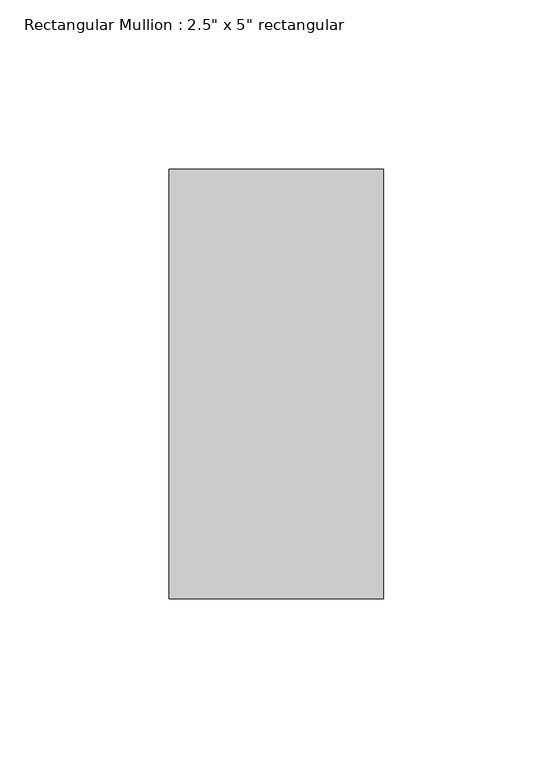
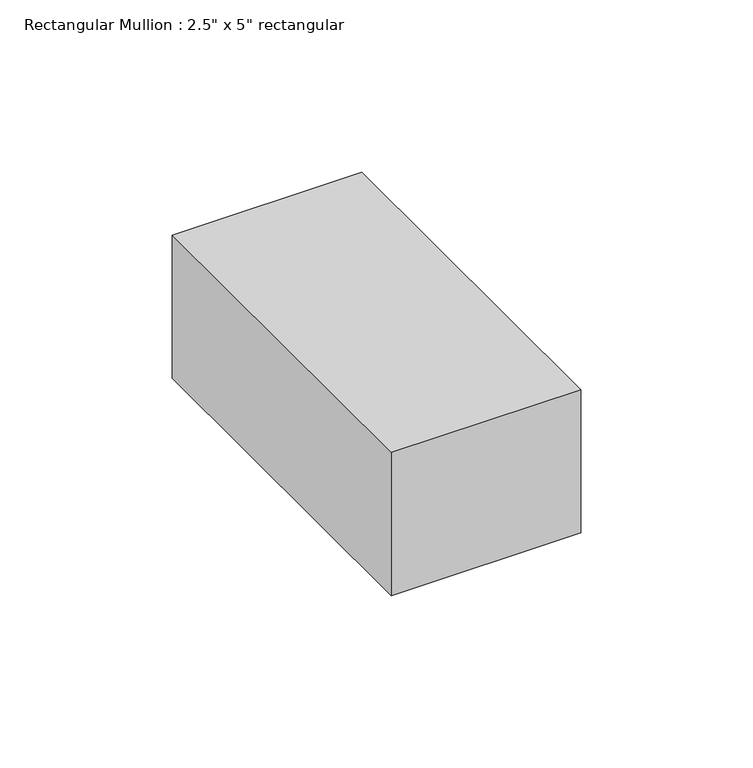
"""IFC4 building model written with IfcOpenShell, lengths in millimetres: member geometry."""

from ifc_helpers import new_model, si_unit, frame, origin, place, context, project, spatial, polyline, outline, extrude, source, transform, mapped, element, save


def member_06be906d(model_context):
    return source(origin(), model_context, "Body", "SweptSolid", [
        extrude(outline(polyline([(31.75, 63.5), (31.75, -63.5), (-31.75, -63.5), (-31.75, 63.5), (31.75, 63.5)])), frame((0.0, 0.0, -50.8), z_axis=(0.0, 0.0, 1.0), x_axis=(1.0, 0.0, 0.0)), (0.0, 0.0, 1.0), 50.8),
    ])


if __name__ == "__main__":
    model = new_model("IFC4")
    model_context = context("Model", 3, world=origin())
    ifc_project = project(units=[si_unit("LENGTHUNIT", "METRE", prefix="MILLI")], contexts=[model_context])
    site = spatial("IfcSite", under=ifc_project)
    building = spatial("IfcBuilding", under=site)
    placement = place(None, origin())
    member_shape = member_06be906d(model_context)
    element("IfcMember", 1, ObjectType="Rectangular Mullion : 2.5\" x 5\" rectangular", at=placement, inside=building, context=model_context, shape_type="MappedRepresentation", body=[
        mapped(member_shape, transform((0.0, 0.0, 0.0), x_axis=(1.0, 0.0, 0.0), y_axis=(0.0, 1.0, 0.0), z_axis=(0.0, 0.0, 1.0))),
    ])
    save(model, "model.ifc")

# Revit data of these elements
# Type "Rectangular Mullion : 2.5\" x 5\" rectangular"
#   built-in parameter 1007304 = 0.416667 (stored number, unit not read)
#   built-in parameter 1007301 = 0.104167 (stored number, unit not read)
#   built-in parameter 1007300 = 0.104167 (stored number, unit not read)
# Element 1 (IfcMember, "Rectangular Mullion : 2.5\" x 5\" rectangular")
#   Materials on its faces: "Aluminum"
# Materials
#   "Aluminum": class "Metal", colour RGB 247 247 247, transparency 0, Description = "Aluminum 6061", Cost = 0
